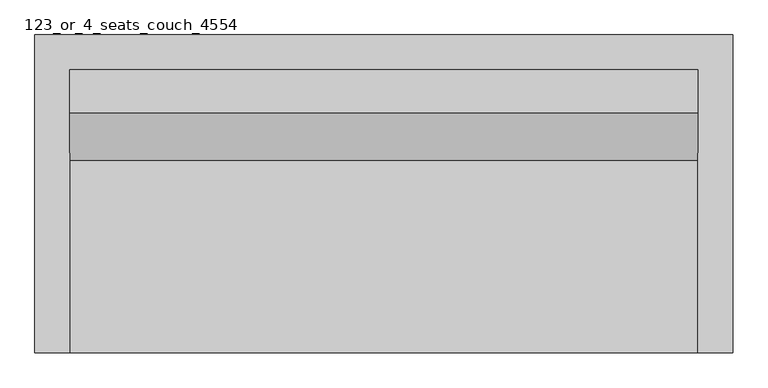
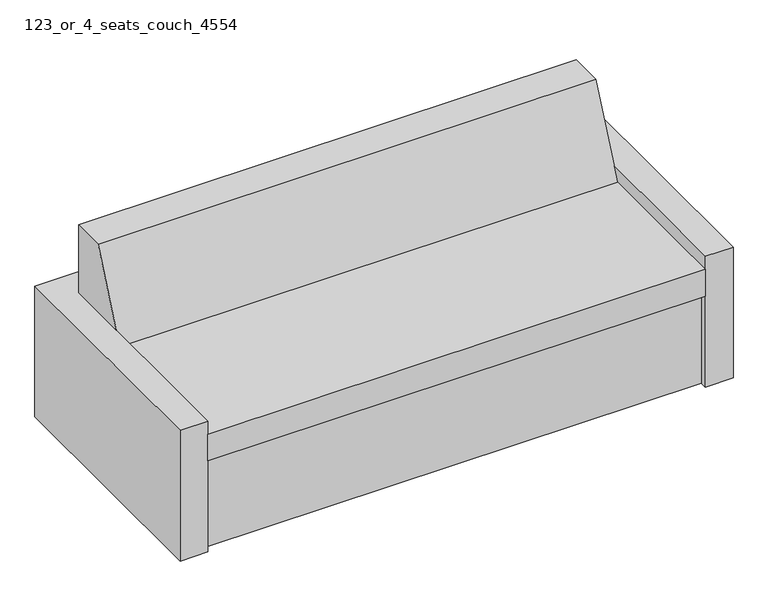
"""IFC4 building model written with IfcOpenShell, lengths in millimetres: furniture geometry, 123_or_4_seats_couch_4554."""

from ifc_helpers import new_model, si_unit, frame, origin, origin_with_axes, place, context, project, spatial, polyline, outline, extrude, source, transform, mapped, element, save


def furniture_123_or_4_seats_couch_4554_e45b83ba(model_context):
    return source(origin(), model_context, "Body", "SweptSolid", [
        extrude(outline(polyline([(-359.4256442, 450.0), (-222.4208629, 760.0), (-100.0, 760.0), (-100.0, 0.0), (-884.6, 0.0), (-884.6, 348.4), (-910.0, 348.4), (-910.0, 450.0), (-359.4256442, 450.0)])), frame((-823.8, 0.0, 0.0), z_axis=(1.0, 0.0, 0.0), x_axis=(0.0, 1.0, 0.0)), (0.0, 0.0, 1.0), 1800.0),
        extrude(outline(polyline([(1076.2, 0.0), (1076.2, -910.0), (976.2, -910.0), (976.2, -100.0), (-823.8, -100.0), (-823.8, -910.0), (-923.8, -910.0), (-923.8, 0.0), (1076.2, 0.0)])), origin_with_axes(), (0.0, 0.0, 1.0), 500.0),
    ])


if __name__ == "__main__":
    model = new_model("IFC4")
    model_context = context("Model", 3, world=origin())
    ifc_project = project(units=[si_unit("LENGTHUNIT", "METRE", prefix="MILLI")], contexts=[model_context])
    site = spatial("IfcSite", under=ifc_project)
    building = spatial("IfcBuilding", under=site)
    placement = place(None, origin())
    furniture_123_or_4_seats_couch_4554_shape = furniture_123_or_4_seats_couch_4554_e45b83ba(model_context)
    element("IfcFurniture", 1, ObjectType="123_or_4_seats_couch_4554", at=placement, inside=building, context=model_context, shape_type="MappedRepresentation", body=[
        mapped(furniture_123_or_4_seats_couch_4554_shape, transform((0.0, 0.0, 0.0), x_axis=(1.0, 0.0, 0.0), y_axis=(0.0, 1.0, 0.0), z_axis=(0.0, 0.0, 1.0))),
    ])
    save(model, "model.ifc")

# Revit data of these elements
# Type "123_or_4_seats_couch_4554"
#   width = 6' - 6.74016"
#   seat height = 1' - 5.71654"
#   height = 2' - 5.92126"
#   depth = 2' - 11.82677"
#   arm height = 1' - 7.68504"
#   arm depth = 0' - 3.93701"
#   Total Seat Room = 5' - 10.86614"
#   Seat Width = 1' - 11.62205"
#   Seat Count = 3
#   Is Mark Visible = yes
#   seat material = Sofa seat
#   arm material = Sofa arm
#   Default Elevation = 0
#   Assembly Code = ""
# Element 1 (IfcFurniture, "123_or_4_seats_couch_4554")
#   Materials on its faces: "Sofa seat", "Sofa arm"
# Materials
#   "Sofa seat": colour RGB 247 247 239, transparency 0
#   "Sofa arm": colour RGB 247 247 239, transparency 0
